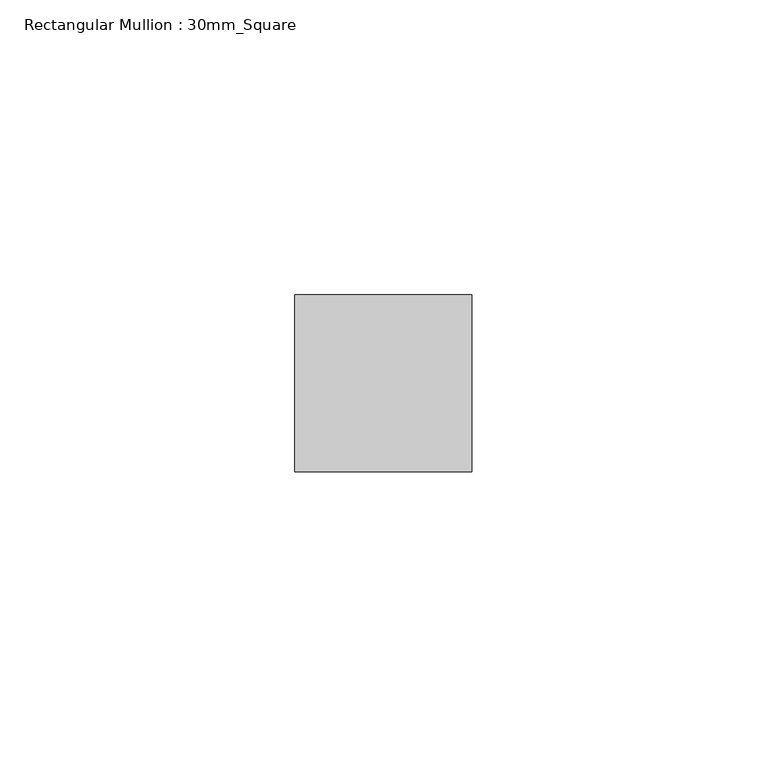
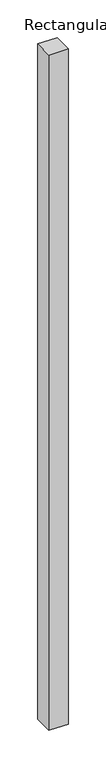
"""IFC4 building model written with IfcOpenShell, lengths in millimetres: member geometry, Rectangular Mullion : 30mm_Square."""

from ifc_helpers import new_model, si_unit, frame, origin, place, context, project, spatial, polyline, outline, extrude, source, transform, mapped, element, save


def rectangular_mullion_30mm_square_9211323b(model_context):
    return source(origin(), model_context, "Body", "SweptSolid", [
        extrude(outline(polyline([(15.0, 15.0), (15.0, -15.0), (-15.0, -15.0), (-15.0, 15.0), (15.0, 15.0)])), frame((0.0, 0.0, -1098.5425256), z_axis=(0.0, 0.0, 1.0), x_axis=(1.0, 0.0, 0.0)), (0.0, 0.0, 1.0), 1098.5425256),
    ])


if __name__ == "__main__":
    model = new_model("IFC4")
    model_context = context("Model", 3, world=origin())
    ifc_project = project(units=[si_unit("LENGTHUNIT", "METRE", prefix="MILLI")], contexts=[model_context])
    site = spatial("IfcSite", under=ifc_project)
    building = spatial("IfcBuilding", under=site)
    placement = place(None, origin())
    rectangular_mullion_30mm_square_shape = rectangular_mullion_30mm_square_9211323b(model_context)
    element("IfcMember", 1, ObjectType="Rectangular Mullion : 30mm_Square", at=placement, inside=building, context=model_context, shape_type="MappedRepresentation", body=[
        mapped(rectangular_mullion_30mm_square_shape, transform((0.0, 0.0, 0.0), x_axis=(1.0, 0.0, 0.0), y_axis=(0.0, 1.0, 0.0), z_axis=(0.0, 0.0, 1.0))),
    ])
    save(model, "model.ifc")

# Revit data of these elements
# Type "Rectangular Mullion : 30mm_Square"
#   Keynote = "H11"
#   built-in parameter 1007304 = 0.0984252 (stored number, unit not read)
#   built-in parameter 1007301 = 0.0492126 (stored number, unit not read)
#   built-in parameter 1007300 = 0.0492126 (stored number, unit not read)
# Element 1 (IfcMember, "Rectangular Mullion : 30mm_Square")
#   Materials on its faces: "Aluminium"
# Materials
#   "Aluminium": class "Metal", colour RGB 247 247 247, transparency 0, Description = "Aluminium 6061", Cost = 0
